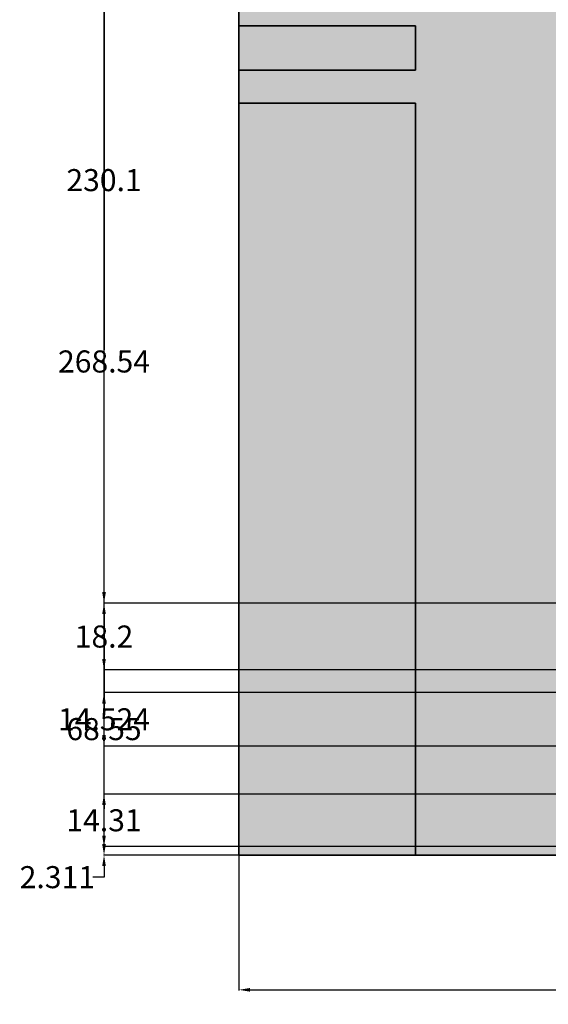
# Model space of a CAD drawing. Units: inches. Extents: x 126 to 726, y 86 to 888.
# Tile 1 of 13: x 126 to 270, y 86 to 354. Entities that reach past the tile are written whole.
import ezdxf

# ---------------------------------------------------------------- set-up
doc = ezdxf.new("R2010")
doc.units = ezdxf.units.IN
doc.header["$MEASUREMENT"] = 0
for name, color, linetype, lineweight in [('A-ANNO-DIMS', 2, 'Continuous', 18), ('A-ELEV', 7, 'Continuous', 35), ('A-ELEV-PATT', 8, 'Continuous', 13)]:
    doc.layers.add(name, color=color, linetype=linetype, lineweight=lineweight)
doc.styles.get("Standard").update_dxf_attribs({"font": 'arial.ttf'})
doc.dimstyles.get("Standard").update_dxf_attribs({"dimtxt": 6, "dimasz": 3, "dimexe": 0.18, "dimexo": 0.0625, "dimgap": 0.09, "dimtad": 0, "dimtih": 1, "dimtoh": 1, "dimdec": 0, "dimzin": 0, "dimdsep": 46, "dimlunit": 3, "dimtxsty": 'Standard', "dimcen": 0.09, "dimadec": 0, "dimazin": 0, "dimtfac": 1, "dimtdec": 0, "dimtofl": 0, "dimtmove": 0, "dimatfit": 3, "dimfxl": 1, "dimtolj": 1, "dimtzin": 0, "dimarcsym": 0})

# ---------------------------------------------------------------- blocks, each defined once
blk = doc.blocks.new('FACADE-STRIP')
for p, q in [((0, 0), (0, 12)), ((0, 12), (48, 12)), ((0, 0), (48, 0))]:
    blk.add_line(p, q)
blk = doc.blocks.new('*D9')
at = {"layer": 'A-ANNO-DIMS', "color": 0, "lineweight": -2, "transparency": 16777216}
for p, q in [((306.84, 373.93), (303.84, 373.93)), ((306.84, 365.49), (306.84, 374.11)), ((360.53, 373.93), (309.84, 373.93)), ((363.53, 365.49), (363.53, 374.11))]:
    blk.add_line(p, q, dxfattribs=at)
at = {"layer": 'A-ANNO-DIMS', "color": 0, "transparency": 16777216}
for points in [[(309.84, 374.43), (309.84, 373.43), (306.84, 373.93)], [(360.53, 374.43), (360.53, 373.43), (363.53, 373.93)]]:
    blk.add_solid(points, dxfattribs=at)
at = {"layer": 'Defpoints', "color": 0, "transparency": 16777216}
for p in [(306.84, 373.93), (306.84, 365.42), (363.53, 365.42)]:
    blk.add_point(p, dxfattribs=at)
at = {"layer": 'A-ANNO-DIMS', "color": 0, "transparency": 16777216, "insert": (235.05, 373.93), "char_height": 6, "attachment_point": 5}
blk.add_mtext('\\A1;DECORATIVE RING MOTIF 57 TYP.', dxfattribs=at)
blk = doc.blocks.new('*D13')
at = {"layer": 'A-ANNO-DIMS', "color": 0, "lineweight": -2, "transparency": 16777216}
for p, q in [((665.97, 642.98), (665.97, 90.21)), ((185.97, 126.98), (185.97, 90.21)), ((188.97, 90.39), (419.15, 90.39)), ((662.97, 90.39), (432.8, 90.39))]:
    blk.add_line(p, q, dxfattribs=at)
at = {"layer": 'A-ANNO-DIMS', "color": 0, "transparency": 16777216}
for points in [[(188.97, 90.89), (188.97, 89.89), (185.97, 90.39)], [(662.97, 90.89), (662.97, 89.89), (665.97, 90.39)]]:
    blk.add_solid(points, dxfattribs=at)
at = {"layer": 'Defpoints', "color": 0, "transparency": 16777216}
for p in [(665.97, 643.04), (185.97, 127.04), (665.97, 90.39)]:
    blk.add_point(p, dxfattribs=at)
at = {"layer": 'A-ANNO-DIMS', "color": 0, "transparency": 16777216, "insert": (425.97, 90.39), "char_height": 6, "attachment_point": 5}
blk.add_mtext('\\A1;480', dxfattribs=at)
blk = doc.blocks.new('*D14')
at = {"layer": 'A-ANNO-DIMS', "color": 0, "lineweight": -2, "transparency": 16777216}
for p, q in [((185.91, 847.04), (149.14, 847.04)), ((149.32, 844.04), (149.32, 490.2)), ((149.32, 130.04), (149.32, 483.89)), ((185.91, 127.04), (149.14, 127.04))]:
    blk.add_line(p, q, dxfattribs=at)
at = {"layer": 'A-ANNO-DIMS', "color": 0, "transparency": 16777216}
for points in [[(148.82, 844.04), (149.82, 844.04), (149.32, 847.04)], [(148.82, 130.04), (149.82, 130.04), (149.32, 127.04)]]:
    blk.add_solid(points, dxfattribs=at)
at = {"layer": 'Defpoints', "color": 0, "transparency": 16777216}
for p in [(149.32, 847.04), (185.97, 847.04), (185.97, 127.04)]:
    blk.add_point(p, dxfattribs=at)
at = {"layer": 'A-ANNO-DIMS', "color": 0, "transparency": 16777216, "insert": (149.32, 487.04), "char_height": 6, "attachment_point": 5}
blk.add_mtext('\\A1;720', dxfattribs=at)
blk = doc.blocks.new('*D15')
at = {"layer": 'A-ANNO-DIMS', "color": 0, "lineweight": -2, "transparency": 16777216}
for p, q in [((299.6, 195.59), (149.14, 195.59)), ((149.32, 192.59), (149.32, 164.47)), ((149.32, 130.04), (149.32, 158.16)), ((185.91, 127.04), (149.14, 127.04))]:
    blk.add_line(p, q, dxfattribs=at)
at = {"layer": 'A-ANNO-DIMS', "color": 0, "transparency": 16777216}
for points in [[(148.82, 192.59), (149.82, 192.59), (149.32, 195.59)], [(148.82, 130.04), (149.82, 130.04), (149.32, 127.04)]]:
    blk.add_solid(points, dxfattribs=at)
at = {"layer": 'Defpoints', "color": 0, "transparency": 16777216}
for p in [(149.32, 195.59), (299.67, 195.59), (185.97, 127.04)]:
    blk.add_point(p, dxfattribs=at)
at = {"layer": 'A-ANNO-DIMS', "color": 0, "transparency": 16777216, "insert": (149.32, 161.31), "char_height": 6, "attachment_point": 5}
blk.add_mtext('\\A1;68.55', dxfattribs=at)
blk = doc.blocks.new('*D16')
at = {"layer": 'A-ANNO-DIMS', "color": 0, "lineweight": -2, "transparency": 16777216}
for p, q in [((299.6, 425.68), (149.14, 425.68)), ((149.32, 422.68), (149.32, 313.79)), ((149.32, 198.59), (149.32, 307.48)), ((299.6, 195.59), (149.14, 195.59))]:
    blk.add_line(p, q, dxfattribs=at)
at = {"layer": 'A-ANNO-DIMS', "color": 0, "transparency": 16777216}
for points in [[(148.82, 422.68), (149.82, 422.68), (149.32, 425.68)], [(148.82, 198.59), (149.82, 198.59), (149.32, 195.59)]]:
    blk.add_solid(points, dxfattribs=at)
at = {"layer": 'Defpoints', "color": 0, "transparency": 16777216}
for p in [(149.32, 425.68), (299.67, 425.68), (299.67, 195.59)]:
    blk.add_point(p, dxfattribs=at)
at = {"layer": 'A-ANNO-DIMS', "color": 0, "transparency": 16777216, "insert": (149.32, 310.64), "char_height": 6, "attachment_point": 5}
blk.add_mtext('\\A1;230.1', dxfattribs=at)
blk = doc.blocks.new('*D18')
at = {"layer": 'A-ANNO-DIMS', "color": 0, "lineweight": -2, "transparency": 16777216}
for p, q in [((431.28, 395.58), (149.14, 395.58)), ((149.32, 392.58), (149.32, 264.47)), ((149.32, 130.04), (149.32, 258.16)), ((185.91, 127.04), (149.14, 127.04))]:
    blk.add_line(p, q, dxfattribs=at)
at = {"layer": 'A-ANNO-DIMS', "color": 0, "transparency": 16777216}
for points in [[(148.82, 392.58), (149.82, 392.58), (149.32, 395.58)], [(148.82, 130.04), (149.82, 130.04), (149.32, 127.04)]]:
    blk.add_solid(points, dxfattribs=at)
at = {"layer": 'Defpoints', "color": 0, "transparency": 16777216}
for p in [(149.32, 395.58), (431.34, 395.58), (185.97, 127.04)]:
    blk.add_point(p, dxfattribs=at)
at = {"layer": 'A-ANNO-DIMS', "color": 0, "transparency": 16777216, "insert": (149.32, 261.31), "char_height": 6, "attachment_point": 5}
blk.add_mtext('\\A1;268.54', dxfattribs=at)
blk = doc.blocks.new('*D30')
at = {"layer": 'A-ANNO-DIMS', "color": 0, "lineweight": -2, "transparency": 16777216}
for p, q in [((299.6, 195.59), (149.14, 195.59)), ((149.32, 192.59), (149.32, 189.64)), ((149.32, 180.39), (149.32, 183.33)), ((326.24, 177.39), (149.14, 177.39))]:
    blk.add_line(p, q, dxfattribs=at)
at = {"layer": 'A-ANNO-DIMS', "color": 0, "transparency": 16777216}
for points in [[(148.82, 192.59), (149.82, 192.59), (149.32, 195.59)], [(148.82, 180.39), (149.82, 180.39), (149.32, 177.39)]]:
    blk.add_solid(points, dxfattribs=at)
at = {"layer": 'Defpoints', "color": 0, "transparency": 16777216}
for p in [(149.32, 195.59), (299.67, 195.59), (326.3, 177.39)]:
    blk.add_point(p, dxfattribs=at)
at = {"layer": 'A-ANNO-DIMS', "color": 0, "transparency": 16777216, "insert": (149.32, 186.49), "char_height": 6, "attachment_point": 5}
blk.add_mtext('\\A1;18.2', dxfattribs=at)
blk = doc.blocks.new('*D37')
at = {"layer": 'A-ANNO-DIMS', "color": 0, "lineweight": -2, "transparency": 16777216}
for p, q in [((307.74, 171.24), (149.14, 171.24)), ((149.32, 168.24), (149.32, 167.13)), ((149.32, 159.71), (149.32, 160.82)), ((307.74, 156.71), (149.14, 156.71))]:
    blk.add_line(p, q, dxfattribs=at)
at = {"layer": 'A-ANNO-DIMS', "color": 0, "transparency": 16777216}
for points in [[(148.82, 168.24), (149.82, 168.24), (149.32, 171.24)], [(148.82, 159.71), (149.82, 159.71), (149.32, 156.71)]]:
    blk.add_solid(points, dxfattribs=at)
at = {"layer": 'Defpoints', "color": 0, "transparency": 16777216}
for p in [(149.32, 171.24), (307.8, 171.24), (307.8, 156.71)]:
    blk.add_point(p, dxfattribs=at)
at = {"layer": 'A-ANNO-DIMS', "color": 0, "transparency": 16777216, "insert": (149.32, 163.98), "char_height": 6, "attachment_point": 5}
blk.add_mtext('\\A1;14.524', dxfattribs=at)
blk = doc.blocks.new('*D79')
at = {"layer": 'A-ANNO-DIMS', "color": 0, "lineweight": -2, "transparency": 16777216}
for p, q in [((149.32, 132.35), (149.32, 135.35)), ((437.91, 129.35), (149.14, 129.35)), ((485.91, 127.04), (149.14, 127.04)), ((149.32, 124.04), (149.32, 121.04)), ((149.32, 121.04), (146.32, 121.04))]:
    blk.add_line(p, q, dxfattribs=at)
at = {"layer": 'A-ANNO-DIMS', "color": 0, "transparency": 16777216}
for points in [[(148.82, 132.35), (149.82, 132.35), (149.32, 129.35)], [(148.82, 124.04), (149.82, 124.04), (149.32, 127.04)]]:
    blk.add_solid(points, dxfattribs=at)
at = {"layer": 'Defpoints', "color": 0, "transparency": 16777216}
for p in [(437.97, 129.35), (149.32, 127.04), (485.97, 127.04)]:
    blk.add_point(p, dxfattribs=at)
at = {"layer": 'A-ANNO-DIMS', "color": 0, "transparency": 16777216, "insert": (136.64, 121.04), "char_height": 6, "attachment_point": 5}
blk.add_mtext('\\A1;2.311', dxfattribs=at)
blk = doc.blocks.new('*D80')
at = {"layer": 'A-ANNO-DIMS', "color": 0, "lineweight": -2, "transparency": 16777216}
for p, q in [((437.91, 143.66), (149.14, 143.66)), ((149.32, 140.66), (149.32, 139.66)), ((149.32, 132.35), (149.32, 133.35)), ((437.91, 129.35), (149.14, 129.35))]:
    blk.add_line(p, q, dxfattribs=at)
at = {"layer": 'A-ANNO-DIMS', "color": 0, "transparency": 16777216}
for points in [[(148.82, 140.66), (149.82, 140.66), (149.32, 143.66)], [(148.82, 132.35), (149.82, 132.35), (149.32, 129.35)]]:
    blk.add_solid(points, dxfattribs=at)
at = {"layer": 'Defpoints', "color": 0, "transparency": 16777216}
for p in [(149.32, 143.66), (437.97, 143.66), (437.97, 129.35)]:
    blk.add_point(p, dxfattribs=at)
at = {"layer": 'A-ANNO-DIMS', "color": 0, "transparency": 16777216, "insert": (149.32, 136.51), "char_height": 6, "attachment_point": 5}
blk.add_mtext('\\A1;14.31', dxfattribs=at)

msp = doc.modelspace()

# ---------------------------------------------------------------- hatches: boundary and pattern name
at = {"layer": 'A-ELEV-PATT'}
h = msp.add_hatch(color=256, dxfattribs=at)
h.dxf.hatch_style = 1
h.paths.add_polyline_path([(437.9749, 499.1312), (485.9749, 499.1312), (485.9749, 501.4423), (437.9749, 501.4423), (437.9749, 513.4423), (485.9749, 513.4423), (485.9749, 515.7534), (437.9749, 515.7534), (437.9749, 527.7534), (485.9749, 527.7534), (485.9749, 530.0646), (437.9749, 530.0646), (437.9749, 542.0646), (485.9749, 542.0646), (485.9749, 544.3757), (437.9749, 544.3757), (437.9749, 556.3757), (485.9749, 556.3757), (485.9749, 558.6868), (437.9749, 558.6868), (437.9749, 570.6868), (485.9749, 570.6868), (485.9749, 572.9979), (437.9749, 572.9979), (437.9749, 584.9979), (485.9749, 584.9979), (485.9749, 587.309), (437.9749, 587.309), (437.9749, 595.0424), (429.9749, 595.0424), (429.9749, 607.0424), (437.9749, 607.0424), (437.9749, 615.9312), (437.9749, 630.2423), (437.9749, 642.2423), (485.9749, 642.2423), (485.9749, 644.5534), (437.9749, 644.5534), (437.9749, 656.5534), (485.9749, 656.5534), (485.9749, 658.8645), (437.9749, 658.8645), (437.9749, 670.8645), (485.9749, 670.8645), (485.9749, 673.1757), (437.9749, 673.1757), (437.9749, 685.1757), (485.9749, 685.1757), (485.9749, 687.4868), (437.9749, 687.4868), (437.9749, 699.4868), (485.9749, 699.4868), (485.9749, 701.7979), (437.9749, 701.7979), (437.9749, 713.7979), (485.9749, 713.7979), (485.9749, 716.109), (437.9749, 716.109), (437.9749, 728.109), (485.9749, 728.109), (485.9749, 730.4201), (437.9749, 730.4201), (437.9749, 742.4201), (485.9749, 742.4201), (485.9749, 744.7312), (437.9749, 744.7312), (437.9749, 756.7312), (485.9749, 756.7312), (485.9749, 759.0423), (437.9749, 759.0423), (437.9749, 771.0423), (485.9749, 771.0423), (485.9749, 773.3534), (437.9749, 773.3534), (437.9749, 785.3534), (485.9749, 785.3534), (485.9749, 787.6645), (437.9749, 787.6645), (437.9749, 799.6645), (485.9749, 799.6645), (485.9749, 801.9756), (437.9749, 801.9756), (437.9749, 811.2868), (485.9749, 811.2868), (485.9749, 813.9756), (437.9749, 813.9756), (437.9749, 825.9756), (485.9749, 825.9756), (485.9749, 835.0424), (233.9749, 835.0424), (233.9749, 606.5846), (185.9749, 606.5846), (185.9749, 597.5846), (233.9749, 597.5846), (233.9749, 585.5846), (185.9749, 585.5846), (185.9749, 580.5846), (233.9749, 580.5846), (233.9749, 568.5846), (185.9749, 568.5846), (185.9749, 563.5846), (431.3386, 563.5846), (431.3386, 545.5846), (233.9749, 545.5846), (233.9749, 413.5846), (431.3386, 413.5846), (431.3386, 395.5846), (185.9749, 395.5846), (185.9749, 386.5846), (233.9749, 386.5846), (233.9749, 374.5846), (185.9749, 374.5846), (185.9749, 369.5846), (233.9749, 369.5846), (233.9749, 357.5846), (185.9749, 357.5846), (185.9749, 352.5846), (233.9749, 352.5846), (233.9749, 340.5846), (185.9749, 340.5846), (185.9749, 331.5846), (233.9749, 331.5846), (233.9749, 127.0424), (485.9749, 127.0424), (485.9749, 129.3535), (437.9749, 129.3535), (437.9749, 141.3535), (485.9749, 141.3535), (485.9749, 143.6646), (437.9749, 143.6646), (437.9749, 155.6646), (485.9749, 155.6646), (485.9749, 157.9757), (437.9749, 157.9757), (437.9749, 169.9757), (485.9749, 169.9757), (485.9749, 172.2868), (437.9749, 172.2868), (437.9749, 184.2868), (485.9749, 184.2868), (485.9749, 186.5979), (437.9749, 186.5979), (437.9749, 198.5979), (485.9749, 198.5979), (485.9749, 200.909), (437.9749, 200.909), (437.9749, 212.909), (485.9749, 212.909), (485.9749, 215.2201), (437.9749, 215.2201), (437.9749, 227.2201), (485.9749, 227.2201), (485.9749, 229.5312), (437.9749, 229.5312), (437.9749, 241.5312), (485.9749, 241.5312), (485.9749, 243.8424), (437.9749, 243.8424), (437.9749, 255.8424), (485.9749, 255.8424), (485.9749, 258.1535), (437.9749, 258.1535), (437.9749, 270.1535), (485.9749, 270.1535), (485.9749, 272.4646), (437.9749, 272.4646), (437.9749, 284.4646), (485.9749, 284.4646), (485.9749, 286.7757), (437.9749, 286.7757), (437.9749, 298.7757), (485.9749, 298.7757), (485.9749, 301.0868), (437.9749, 301.0868), (437.9749, 313.0868), (485.9749, 313.0868), (485.9749, 315.3979), (437.9749, 315.3979), (437.9749, 327.3979), (485.9749, 327.3979), (485.9749, 329.709), (437.9749, 329.709), (437.9749, 341.709), (485.9749, 341.709), (485.9749, 344.0201), (437.9749, 344.0201), (437.9749, 355.0424), (429.9749, 355.0424), (429.9749, 367.0424), (437.9749, 367.0424), (437.9749, 372.6423), (437.9749, 386.9535), (437.9749, 401.2646), (437.9749, 413.2646), (485.9749, 413.2646), (485.9749, 415.5757), (437.9749, 415.5757), (437.9749, 427.5757), (485.9749, 427.5757), (485.9749, 429.8868), (437.9749, 429.8868), (437.9749, 441.8868), (485.9749, 441.8868), (485.9749, 444.1979), (437.9749, 444.1979), (437.9749, 456.1979), (485.9749, 456.1979), (485.9749, 458.509), (437.9749, 458.509), (437.9749, 470.509), (485.9749, 470.509), (485.9749, 472.8201), (437.9749, 472.8201), (437.9749, 484.8201), (485.9749, 484.8201), (485.9749, 487.1312), (437.9749, 487.1312)])
h.paths.add_polyline_path([(299.6658, 533.6845), (371.6658, 533.6845), (371.6658, 425.6845), (299.6658, 425.6845)], flags=16)
h.paths.add_polyline_path([(308.6658, 524.6845), (362.6658, 524.6845), (362.6658, 434.6845), (308.6658, 434.6845)], flags=0)
h.paths.add_polyline_path([(317.7956, 603.3211, -0.4129833), (306.8418, 614.321, -0.94403766), (328.769, 615.5845, -0.04423165), (330.7031, 615.4048, -0.89973713), (352.5798, 615.6161, -0.4129833), (363.5336, 604.6162, -0.94403766), (341.6064, 603.3528, -0.04423165), (339.6723, 603.5324, -0.89973713)], flags=16)
h.paths.add_polyline_path([(319.7228, 604.5846, -0.02633223), (319.7726, 605.5306, -0.47905713), (308.8418, 614.321, -1), (326.8418, 614.321, -0.02633223), (326.7919, 613.375, -0.17413188), (332.826, 612.5948, -0.04918553), (332.6526, 614.3527, -1), (350.6526, 614.3527, -0.02633223), (350.6028, 613.4067, -0.47905713), (361.5336, 604.6162, -1), (343.5336, 604.6162, -0.02633223), (343.5834, 605.5622, -0.17413188), (337.5494, 606.3424, -0.04918553), (337.7228, 604.5846, -1)], flags=0)
h.paths.add_polyline_path([(328.769, 355.6561, -0.04423165), (330.7031, 355.4765, -0.89973713), (352.5798, 355.6878, -0.4129833), (363.5336, 344.6879, -0.94403766), (341.6064, 343.4244, -0.04423165), (339.6723, 343.604, -0.89973713), (317.7956, 343.3927, -0.4129833), (306.8418, 354.3926, -0.94403766)], flags=16)
h.paths.add_polyline_path([(326.8418, 354.3926, -0.02633223), (326.7919, 353.4466, -0.17413188), (332.826, 352.6664, -0.04918553), (332.6526, 354.4243, -1), (350.6526, 354.4243, -0.02633223), (350.6028, 353.4783, -0.47905713), (361.5336, 344.6879, -1), (343.5336, 344.6879, -0.02633223), (343.5834, 345.6339, -0.17413188), (337.5494, 346.4141, -0.04918553), (337.7228, 344.6562, -1), (319.7228, 344.6562, -0.02633223), (319.7726, 345.6022, -0.47905713), (308.8418, 354.3926, -1)], flags=0)
h.paths.add_polyline_path([(299.3189, 655.3527), (299.3189, 763.3527), (371.3189, 763.3527), (371.3189, 655.3527)], flags=16)
h.paths.add_polyline_path([(308.3189, 664.3527), (308.3189, 754.3527), (362.3189, 754.3527), (362.3189, 664.3527)], flags=0)
h.paths.add_polyline_path([(299.6658, 303.5875), (371.6658, 303.5875), (371.6658, 195.5875), (299.6658, 195.5875)], flags=16)
h.paths.add_polyline_path([(308.6658, 294.5875), (362.6658, 294.5875), (362.6658, 204.5875), (308.6658, 204.5875)], flags=0)
h.paths.add_polyline_path([(326.3038, 177.3867), (346.055, 177.3867, -0.41421356), (349.055, 174.3867), (349.055, 171.2378), (363.489, 171.2378, -0.41421356), (366.489, 168.2378), (366.489, 159.7133, -0.41421356), (363.489, 156.7133), (343.7379, 156.7133, -0.41421356), (340.7379, 159.7133), (340.7379, 162.8622), (330.5504, 162.8622), (330.5504, 159.7133, -0.41421356), (327.5504, 156.7133), (307.7992, 156.7133, -0.41421356), (304.7992, 159.7133), (304.7992, 168.2378, -0.41421356), (307.7992, 171.2378), (323.3038, 171.2378), (323.3038, 174.3867, -0.41421356)], flags=16)
h.paths.add_polyline_path([(326.3038, 175.3867), (346.055, 175.3867, -0.41421356), (347.055, 174.3867), (347.055, 169.2378), (363.489, 169.2378, -0.41421356), (364.489, 168.2378), (364.489, 159.7133, -0.41421356), (363.489, 158.7133), (343.7379, 158.7133, -0.41421356), (342.7379, 159.7133), (342.7379, 164.8622), (328.5504, 164.8622), (328.5504, 159.7133, -0.41421356), (327.5504, 158.7133), (307.7992, 158.7133, -0.41421356), (306.7992, 159.7133), (306.7992, 168.2378, -0.41421356), (307.7992, 169.2378), (325.3038, 169.2378), (325.3038, 174.3867, -0.41421356)], flags=0)
h = msp.add_hatch(dxfattribs=at)
h.set_pattern_fill('GRAVEL', color=256, scale=40)
h.paths.add_polyline_path([(437.9749, 642.2423), (485.9749, 642.2423), (485.9749, 644.5534), (437.9749, 644.5534), (437.9749, 656.5534), (485.9749, 656.5534), (485.9749, 658.8645), (437.9749, 658.8645), (437.9749, 670.8645), (485.9749, 670.8645), (485.9749, 673.1757), (437.9749, 673.1757), (437.9749, 685.1757), (485.9749, 685.1757), (485.9749, 687.4868), (437.9749, 687.4868), (437.9749, 699.4868), (485.9749, 699.4868), (485.9749, 701.7979), (437.9749, 701.7979), (437.9749, 713.7979), (485.9749, 713.7979), (485.9749, 716.109), (437.9749, 716.109), (437.9749, 728.109), (485.9749, 728.109), (485.9749, 730.4201), (437.9749, 730.4201), (437.9749, 742.4201), (485.9749, 742.4201), (485.9749, 744.7312), (437.9749, 744.7312), (437.9749, 756.7312), (485.9749, 756.7312), (485.9749, 759.0423), (437.9749, 759.0423), (437.9749, 771.0423), (485.9749, 771.0423), (485.9749, 773.3534), (437.9749, 773.3534), (437.9749, 785.3534), (485.9749, 785.3534), (485.9749, 787.6645), (437.9749, 787.6645), (437.9749, 799.6645), (485.9749, 799.6645), (485.9749, 801.9756), (437.9749, 801.9756), (437.9749, 811.2868), (485.9749, 811.2868), (485.9749, 813.9756), (437.9749, 813.9756), (437.9749, 825.9756), (485.9749, 825.9756), (485.9749, 835.0424), (233.9749, 835.0424), (233.9749, 606.5846), (185.9749, 606.5846), (185.9749, 597.5846), (233.9749, 597.5846), (233.9749, 585.5846), (185.9749, 585.5846), (185.9749, 580.5846), (233.9749, 580.5846), (233.9749, 568.5846), (185.9749, 568.5846), (185.9749, 563.5846), (431.3386, 563.5846), (431.3386, 545.5846), (233.9749, 545.5846), (233.9749, 413.5846), (431.3386, 413.5846), (431.3386, 395.5846), (185.9749, 395.5846), (185.9749, 386.5846), (233.9749, 386.5846), (233.9749, 374.5846), (185.9749, 374.5846), (185.9749, 369.5846), (233.9749, 369.5846), (233.9749, 357.5846), (185.9749, 357.5846), (185.9749, 352.5846), (233.9749, 352.5846), (233.9749, 340.5846), (185.9749, 340.5846), (185.9749, 331.5846), (233.9749, 331.5846), (233.9749, 127.0424), (485.9749, 127.0424), (485.9749, 129.3535), (437.9749, 129.3535), (437.9749, 141.3535), (485.9749, 141.3535), (485.9749, 143.6646), (437.9749, 143.6646), (437.9749, 155.6646), (485.9749, 155.6646), (485.9749, 157.9757), (437.9749, 157.9757), (437.9749, 169.9757), (485.9749, 169.9757), (485.9749, 172.2868), (437.9749, 172.2868), (437.9749, 184.2868), (485.9749, 184.2868), (485.9749, 186.5979), (437.9749, 186.5979), (437.9749, 198.5979), (485.9749, 198.5979), (485.9749, 200.909), (437.9749, 200.909), (437.9749, 212.909), (485.9749, 212.909), (485.9749, 215.2201), (437.9749, 215.2201), (437.9749, 227.2201), (485.9749, 227.2201), (485.9749, 229.5312), (437.9749, 229.5312), (437.9749, 241.5312), (485.9749, 241.5312), (485.9749, 243.8424), (437.9749, 243.8424), (437.9749, 255.8424), (485.9749, 255.8424), (485.9749, 258.1535), (437.9749, 258.1535), (437.9749, 270.1535), (485.9749, 270.1535), (485.9749, 272.4646), (437.9749, 272.4646), (437.9749, 284.4646), (485.9749, 284.4646), (485.9749, 286.7757), (437.9749, 286.7757), (437.9749, 298.7757), (485.9749, 298.7757), (485.9749, 301.0868), (437.9749, 301.0868), (437.9749, 313.0868), (485.9749, 313.0868), (485.9749, 315.3979), (437.9749, 315.3979), (437.9749, 327.3979), (485.9749, 327.3979), (485.9749, 329.709), (437.9749, 329.709), (437.9749, 341.709), (485.9749, 341.709), (485.9749, 344.0201), (437.9749, 344.0201), (437.9749, 355.0424), (429.9749, 355.0424), (429.9749, 367.0424), (437.9749, 367.0424), (437.9749, 372.6423), (437.9749, 386.9535), (437.9749, 401.2646), (437.9749, 413.2646), (485.9749, 413.2646), (485.9749, 415.5757), (437.9749, 415.5757), (437.9749, 427.5757), (485.9749, 427.5757), (485.9749, 429.8868), (437.9749, 429.8868), (437.9749, 441.8868), (485.9749, 441.8868), (485.9749, 444.1979), (437.9749, 444.1979), (437.9749, 456.1979), (485.9749, 456.1979), (485.9749, 458.509), (437.9749, 458.509), (437.9749, 470.509), (485.9749, 470.509), (485.9749, 472.8201), (437.9749, 472.8201), (437.9749, 484.8201), (485.9749, 484.8201), (485.9749, 487.1312), (437.9749, 487.1312), (437.9749, 499.1312), (485.9749, 499.1312), (485.9749, 501.4423), (437.9749, 501.4423), (437.9749, 513.4423), (485.9749, 513.4423), (485.9749, 515.7534), (437.9749, 515.7534), (437.9749, 527.7534), (485.9749, 527.7534), (485.9749, 530.0646), (437.9749, 530.0646), (437.9749, 542.0646), (485.9749, 542.0646), (485.9749, 544.3757), (437.9749, 544.3757), (437.9749, 556.3757), (485.9749, 556.3757), (485.9749, 558.6868), (437.9749, 558.6868), (437.9749, 570.6868), (485.9749, 570.6868), (485.9749, 572.9979), (437.9749, 572.9979), (437.9749, 584.9979), (485.9749, 584.9979), (485.9749, 587.309), (437.9749, 587.309), (437.9749, 595.0424), (429.9749, 595.0424), (429.9749, 607.0424), (437.9749, 607.0424), (437.9749, 615.9312), (437.9749, 630.2423)])
h.paths.add_polyline_path([(371.3189, 655.3527), (299.3189, 655.3527), (299.3189, 763.3527), (371.3189, 763.3527)], flags=16)
h.paths.add_polyline_path([(363.5336, 604.6162, -0.94403766), (341.6064, 603.3528, -0.04423165), (339.6723, 603.5324, -0.89973713), (317.7956, 603.3211, -0.4129833), (306.8418, 614.321, -0.94403766), (328.769, 615.5845, -0.04423165), (330.7031, 615.4048, -0.89973713), (352.5798, 615.6161, -0.4129833)], flags=16)
h.paths.add_polyline_path([(361.5336, 604.6162, -1), (343.5336, 604.6162, -0.02633223), (343.5834, 605.5622, -0.17413188), (337.5494, 606.3424, -0.04918553), (337.7228, 604.5846, -1), (319.7228, 604.5846, -0.02633223), (319.7726, 605.5306, -0.47905713), (308.8418, 614.321, -1), (326.8418, 614.321, -0.02633223), (326.7919, 613.375, -0.17413188), (332.826, 612.5948, -0.04918553), (332.6526, 614.3527, -1), (350.6526, 614.3527, -0.02633223), (350.6028, 613.4067, -0.47905713)], flags=0)
h.paths.add_polyline_path([(362.3189, 664.3527), (308.3189, 664.3527), (308.3189, 754.3527), (362.3189, 754.3527)], flags=0)
h.paths.add_polyline_path([(371.6658, 533.6845), (371.6658, 425.6845), (299.6658, 425.6845), (299.6658, 533.6845)], flags=16)
h.paths.add_polyline_path([(362.6658, 524.6845), (362.6658, 434.6845), (308.6658, 434.6845), (308.6658, 524.6845)], flags=0)
h.paths.add_polyline_path([(352.5798, 355.6878, -0.4129833), (363.5336, 344.6879, -0.94403766), (341.6064, 343.4244, -0.04423165), (339.6723, 343.604, -0.89973713), (317.7956, 343.3927, -0.4129833), (306.8418, 354.3926, -0.94403766), (328.769, 355.6561, -0.04423165), (330.7031, 355.4765, -0.89973713)], flags=16)
h.paths.add_polyline_path([(350.6526, 354.4243, -0.02633223), (350.6028, 353.4783, -0.47905713), (361.5336, 344.6879, -1), (343.5336, 344.6879, -0.02633223), (343.5834, 345.6339, -0.17413188), (337.5494, 346.4141, -0.04918553), (337.7228, 344.6562, -1), (319.7228, 344.6562, -0.02633223), (319.7726, 345.6022, -0.47905713), (308.8418, 354.3926, -1), (326.8418, 354.3926, -0.02633223), (326.7919, 353.4466, -0.17413188), (332.826, 352.6664, -0.04918553), (332.6526, 354.4243, -1)], flags=0)
h.paths.add_polyline_path([(371.6658, 303.5875), (371.6658, 195.5875), (299.6658, 195.5875), (299.6658, 303.5875)], flags=16)
h.paths.add_polyline_path([(362.6658, 294.5875), (362.6658, 204.5875), (308.6658, 204.5875), (308.6658, 294.5875)], flags=0)
h.paths.add_polyline_path([(346.055, 177.3867, -0.41421356), (349.055, 174.3867), (349.055, 171.2378), (363.489, 171.2378, -0.41421356), (366.489, 168.2378), (366.489, 159.7133, -0.41421356), (363.489, 156.7133), (343.7379, 156.7133, -0.41421356), (340.7379, 159.7133), (340.7379, 162.8622), (330.5504, 162.8622), (330.5504, 159.7133, -0.41421356), (327.5504, 156.7133), (307.7992, 156.7133, -0.41421356), (304.7992, 159.7133), (304.7992, 168.2378, -0.41421356), (307.7992, 171.2378), (323.3038, 171.2378), (323.3038, 174.3867, -0.41421356), (326.3038, 177.3867)], flags=16)
h.paths.add_polyline_path([(346.055, 175.3867, -0.41421356), (347.055, 174.3867), (347.055, 169.2378), (363.489, 169.2378, -0.41421356), (364.489, 168.2378), (364.489, 159.7133, -0.41421356), (363.489, 158.7133), (343.7379, 158.7133, -0.41421356), (342.7379, 159.7133), (342.7379, 164.8622), (328.5504, 164.8622), (328.5504, 159.7133, -0.41421356), (327.5504, 158.7133), (307.7992, 158.7133, -0.41421356), (306.7992, 159.7133), (306.7992, 168.2378, -0.41421356), (307.7992, 169.2378), (325.3038, 169.2378), (325.3038, 174.3867, -0.41421356), (326.3038, 175.3867)], flags=0)
h = msp.add_hatch(color=256, dxfattribs=at)
h.dxf.hatch_style = 1
h.paths.add_polyline_path([(233.9749, 331.5846), (185.9749, 331.5846), (185.9749, 127.0424), (233.9749, 127.0424)])
h.paths.add_polyline_path([(233.9749, 352.5846), (185.9749, 352.5846), (185.9749, 340.5846), (233.9749, 340.5846)])
h.paths.add_polyline_path([(233.9749, 369.5846), (185.9749, 369.5846), (185.9749, 357.5846), (233.9749, 357.5846)])
h.paths.add_polyline_path([(233.9749, 386.5846), (185.9749, 386.5846), (185.9749, 374.5846), (233.9749, 374.5846)])

# ---------------------------------------------------------------- linework, layer by layer
at = {"layer": 'A-ELEV'}
for p, q in [((185.9749, 847.0424), (185.9749, 127.0424)), ((185.9749, 331.5846), (233.9749, 331.5846)), ((233.9749, 331.5846), (233.9749, 127.0424)), ((185.9749, 127.0424), (660.0469, 127.0424))]:
    msp.add_line(p, q, dxfattribs=at)

# ---------------------------------------------------------------- block references
at = {"layer": 'A-ELEV', "rotation": 180}
msp.add_blockref('FACADE-STRIP', (233.9748, 352.585), dxfattribs=at)

# ---------------------------------------------------------------- dimensions: what is measured, and where the dimension line sits
at = {"layer": 'A-ANNO-DIMS'}
for base, p1, p2, override, picture, middle in [((149.3249, 847.0424), (185.9749, 127.0424), (185.9749, 847.0424), {"dimdec": 0, "dimlfac": 1, "dimrnd": 0, "dimzin": 0, "dimdsep": 46, "dimlunit": 2}, '*D14', (149.3249, 487.0424)), ((149.3249, 425.6845), (299.6658, 195.5875), (299.6658, 425.6845), {"dimdec": 1, "dimlfac": 1, "dimrnd": 0, "dimzin": 0, "dimdsep": 46, "dimlunit": 2}, '*D16', (149.3249, 310.636)), ((149.3249, 395.5846), (185.9749, 127.0424), (431.3386, 395.5846), {"dimdec": 2, "dimlfac": 1, "dimrnd": 0, "dimzin": 0, "dimdsep": 46, "dimlunit": 2}, '*D18', (149.3249, 261.3135)), ((149.3249, 195.5875), (185.9749, 127.0424), (299.6658, 195.5875), {"dimdec": 2, "dimlfac": 1, "dimrnd": 0, "dimzin": 0, "dimdsep": 46, "dimlunit": 2}, '*D15', (149.3249, 161.3149)), ((149.3249, 195.5875), (326.3038, 177.3867), (299.6658, 195.5875), {"dimdec": 1, "dimlfac": 1, "dimrnd": 0, "dimzin": 0, "dimdsep": 46, "dimlunit": 2}, '*D30', (149.3249, 186.4871)), ((149.32491, 171.23781), (307.79919, 156.71334), (307.79919, 171.23781), {"dimdec": 3, "dimlfac": 1, "dimrnd": 0, "dimzin": 0, "dimdsep": 46, "dimlunit": 2}, '*D37', (149.32491, 163.97557)), ((149.3249, 143.6646), (437.9749, 129.3535), (437.9749, 143.6646), {"dimdec": 2, "dimlfac": 1, "dimrnd": 0, "dimzin": 0, "dimdsep": 46, "dimlunit": 2}, '*D80', (149.3249, 136.509)), ((149.3249, 127.0424), (437.9749, 129.3535), (485.9749, 127.0424), {"dimdec": 3, "dimlfac": 1, "dimrnd": 0, "dimzin": 0, "dimdsep": 46, "dimlunit": 2}, '*D79', (136.6394, 121.0424))]:
    dim = msp.add_linear_dim(base=base, p1=p1, p2=p2, angle=90, dimstyle='Standard', override=override, dxfattribs=at)
    dim.commit()
    dim.dimension.update_dxf_attribs({"geometry": picture, "text_midpoint": middle})
dim = msp.add_linear_dim(base=(665.9749, 90.3924), p1=(185.9749, 127.0424), p2=(665.9749, 643.0424), dimstyle='Standard', override={"dimdec": 0, "dimlfac": 1, "dimrnd": 0, "dimzin": 0, "dimdsep": 46, "dimlunit": 2}, dxfattribs=at)
dim.commit()
dim.dimension.update_dxf_attribs({"geometry": '*D13', "text_midpoint": (425.9749, 90.3924)})
dim = msp.add_linear_dim(base=(306.8418, 373.9281), p1=(363.5336, 365.4243), p2=(306.8418, 365.4243), angle=180, text='DECORATIVE RING MOTIF <> TYP.', dimstyle='Standard', override={"dimdec": 0, "dimlfac": 1, "dimrnd": 0, "dimzin": 0, "dimdsep": 46, "dimlunit": 2}, dxfattribs=at)
dim.commit()
dim.dimension.update_dxf_attribs({"geometry": '*D9', "text_midpoint": (235.0465, 373.9281)})

doc.saveas('drawing.dxf')
